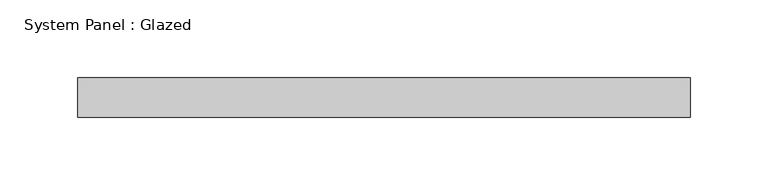
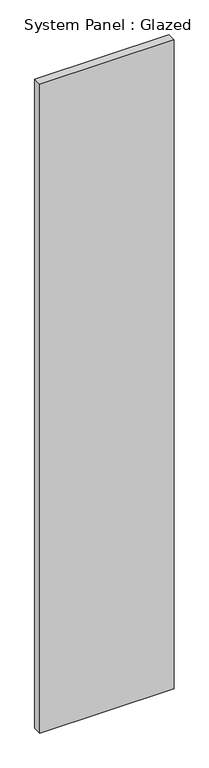
"""IFC4 building model written with IfcOpenShell, lengths in millimetres: plate geometry, System Panel : Glazed."""

from ifc_helpers import new_model, si_unit, origin, origin_with_axes, place, context, project, spatial, polyline, outline, extrude, source, transform, mapped, element, save


def system_panel_glazed_f3f5655f(model_context):
    return source(origin(), model_context, "Body", "SweptSolid", [
        extrude(outline(polyline([(196.85, 19.05), (-196.85, 19.05), (-196.85, 44.45), (196.85, 44.45), (196.85, 19.05)])), origin_with_axes(), (0.0, 0.0, 1.0), 2006.6),
    ])


if __name__ == "__main__":
    model = new_model("IFC4")
    model_context = context("Model", 3, world=origin())
    ifc_project = project(units=[si_unit("LENGTHUNIT", "METRE", prefix="MILLI")], contexts=[model_context])
    site = spatial("IfcSite", under=ifc_project)
    building = spatial("IfcBuilding", under=site)
    placement = place(None, origin())
    system_panel_glazed_shape = system_panel_glazed_f3f5655f(model_context)
    element("IfcPlate", 1, ObjectType="System Panel : Glazed", at=placement, inside=building, context=model_context, shape_type="MappedRepresentation", body=[
        mapped(system_panel_glazed_shape, transform((0.0, 0.0, 0.0), x_axis=(1.0, 0.0, 0.0), y_axis=(0.0, 1.0, 0.0), z_axis=(0.0, 0.0, 1.0))),
    ])
    save(model, "model.ifc")

# Revit data of these elements
# Type "System Panel : Glazed"
#   Construction Type Id = "GSP4R"
#   Analytic Construction = "1/8 in Pilkington single glazing"
#   Visual Light Transmittance = 0.9
#   Solar Heat Gain Coefficient = 0.86
#   Heat Transfer Coefficient (U) = 1.18115 BTU/(h·ft²·°F)
#   Define Thermal Properties by = 1
# Element 1 (IfcPlate, "System Panel : Glazed")
#   Materials on its faces: "Glass"
# Materials
#   "Glass": class "Glass", colour RGB 0 128 192, transparency 0.75, Description = "Soda Lime Glass", Cost = 0
